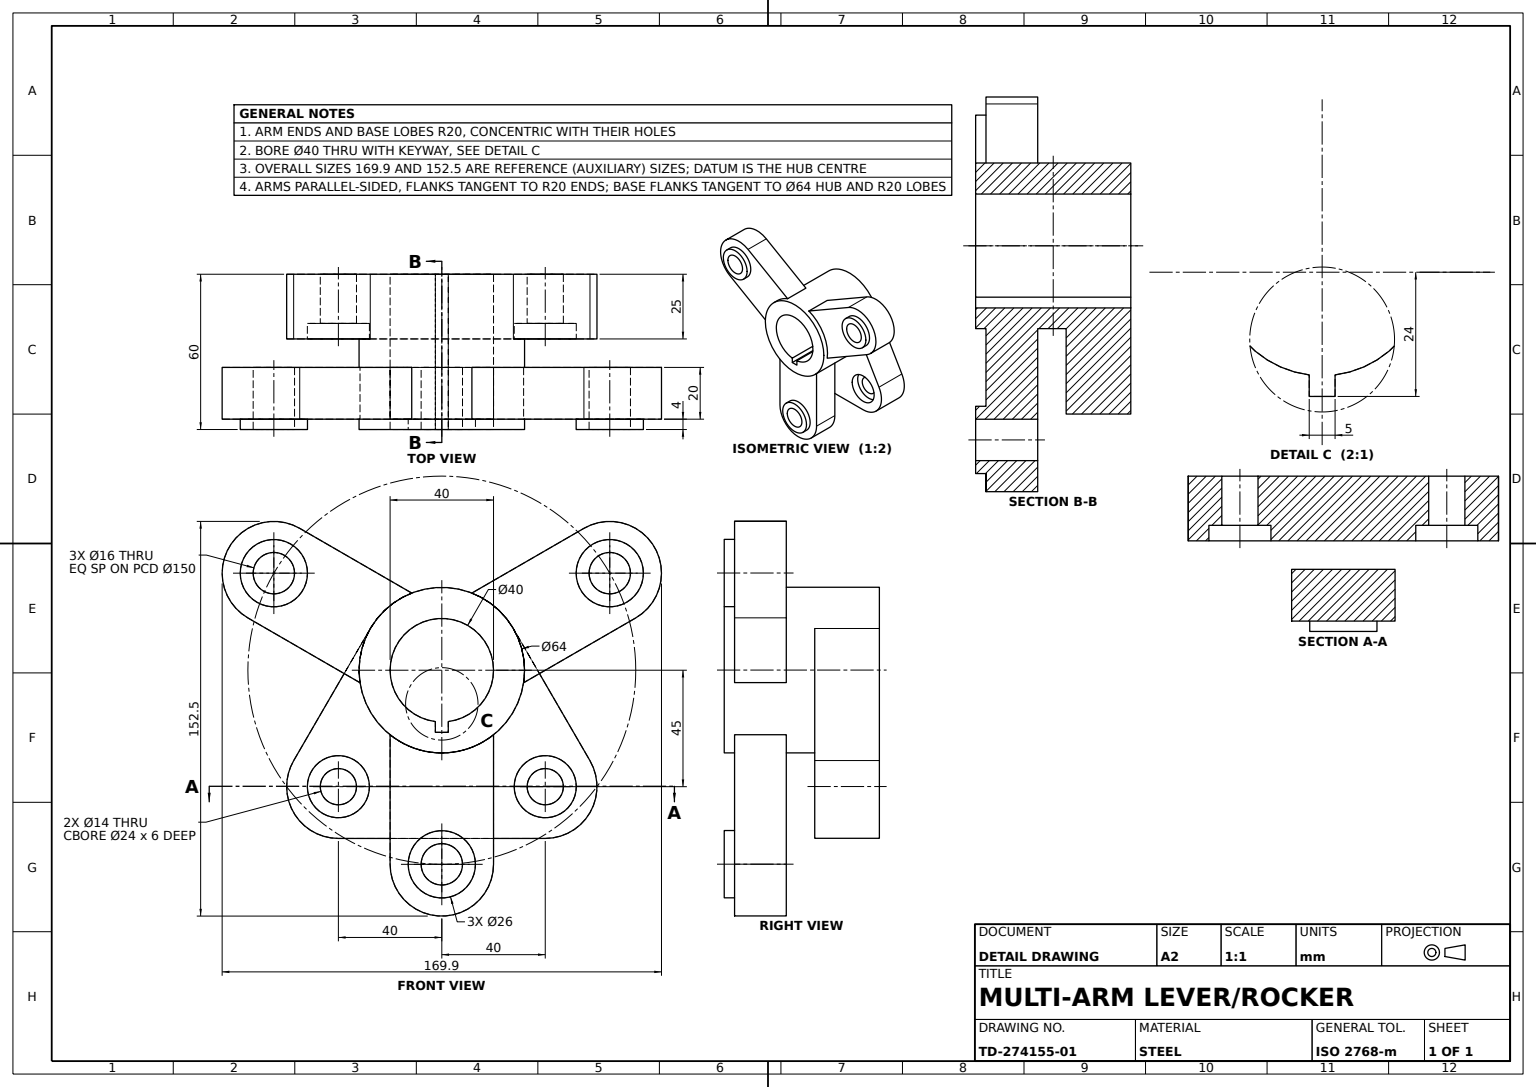
from build123d import *

# Parameters (mm, degrees)
BASE_BLOCK_DEPTH            = 25
HUB_SKETCH_64_R             = 32
HUB_64_DEPTH                = 31
THREE_START                 = -20
THREE_ARMS_120DEG_DEPTH     = 20
HUB_COLLAR_SKETCH_64_R      = 32
HUB_COLLAR_64X4_DEPTH       = 4
BOLT_BOSSES_SKETCH_3X_13_R  = 13
BOLT_BOSSES_3X_13_DEPTH     = 4
BOLT_HOLES_SKETCH_3X_8_R    = 8
BOLT_HOLES_3X_8_DEPTH       = 25
KEYED_BORE_24_DEPTH         = 80
COUNTERBORE_SKETCH_2X_12_R  = 12
COUNTERBORES_2X_12X6_DEPTH  = 6
THROUGH_HOLES_SKETCH_2X_7_R = 7
THROUGH_HOLES_2X_7_DEPTH    = 50


with BuildPart() as part:
    # Base Block Sketch → Base Block (new body)
    with BuildSketch(Plane.XY):
        with BuildLine():
            Line((-57.296551724, -34.95862069), (-27.674482759, 16.066206897))
            ThreePointArc((-27.674482759, 16.066206897), (0, 32), (27.674482759, 16.066206897))
            Line((27.674482759, 16.066206897), (57.296551724, -34.95862069))
            ThreePointArc((57.296551724, -34.95862069), (57.332449137, -54.979288897), (40, -65))
            Line((40, -65), (-40, -65))
            ThreePointArc((-40, -65), (-57.332449137, -54.979288897), (-57.296551724, -34.95862069))
        make_face()
    extrude(amount=BASE_BLOCK_DEPTH)

    # Hub Sketch _64 → Hub _64 (add)
    with BuildSketch(Plane.XY.offset(25)):
        with Locations(Location((0, 0, 0), (0, 0, 149.863023681))):
            Circle(HUB_SKETCH_64_R)
    extrude(amount=HUB_64_DEPTH)

    # Three Arms Sketch → Three Arms 120deg (add)
    with BuildSketch(Plane.XY.offset(56).offset(THREE_START)):
        with BuildLine():
            Line((-20, -75), (-20, -24.979991994))
            ThreePointArc((-20, -24.979991994), (0, -32), (20, -24.979991994))
            Line((20, -24.979991994), (20, -75))
            ThreePointArc((20, -75), (0, -95), (-20, -75))
        make_face()
        with BuildLine():
            Line((-11.633307653, 29.810504072), (-54.951905284, 54.820508076))
            ThreePointArc((-54.951905284, 54.820508076), (-82.27241336, 47.5), (-74.951905284, 20.179491924))
            Line((-74.951905284, 20.179491924), (-31.633307653, -4.830512079))
            ThreePointArc((-31.633307653, -4.830512079), (-27.712812921, 16), (-11.633307653, 29.810504072))
        make_face()
        with BuildLine():
            Line((17.280738855, 33.071049997), (54.951905284, 54.820508076))
            ThreePointArc((54.951905284, 54.820508076), (82.27146994, 47.501633873), (74.955172941, 20.181378918))
            Line((74.955172941, 20.181378918), (37.758368932, -1.303564067))
            Line((37.758368932, -1.303564067), (31.631479851, -4.842466563))
            ThreePointArc((31.631479851, -4.842466563), (27.715835779, 15.994763115), (11.633307653, 29.810504072))
            Line((11.633307653, 29.810504072), (17.280738855, 33.071049997))
        make_face()
    extrude(amount=THREE_ARMS_120DEG_DEPTH)

    # Hub Collar Sketch _64 → Hub Collar _64x4 (add)
    with BuildSketch(Plane.XY.offset(56)):
        with Locations(Location((0, 0, 0), (0, 0, 149.863023681))):
            Circle(HUB_COLLAR_SKETCH_64_R)
    extrude(amount=HUB_COLLAR_64X4_DEPTH)

    # Bolt Bosses Sketch 3x_13 → Bolt Bosses 3x_13 (add)
    with BuildSketch(Plane.XY.offset(56)):
        with Locations((-64.951905284, 37.5)):
            Circle(BOLT_BOSSES_SKETCH_3X_13_R)
        with Locations((64.951905284, 37.5)):
            Circle(BOLT_BOSSES_SKETCH_3X_13_R)
        with Locations((0, -75)):
            Circle(BOLT_BOSSES_SKETCH_3X_13_R)
    extrude(amount=BOLT_BOSSES_3X_13_DEPTH)

    # Bolt Holes Sketch 3x_8 → Bolt Holes 3x_8 (cut)
    with BuildSketch(Plane.XY.offset(60)):
        with Locations((-64.951905284, 37.5)):
            Circle(BOLT_HOLES_SKETCH_3X_8_R)
        with Locations((64.951905284, 37.5)):
            Circle(BOLT_HOLES_SKETCH_3X_8_R)
        with Locations((0, -75)):
            Circle(BOLT_HOLES_SKETCH_3X_8_R)
    extrude(amount=-BOLT_HOLES_3X_8_DEPTH, mode=Mode.SUBTRACT)

    # Keyed Bore Sketch _24 → Keyed Bore _24 (cut)
    with BuildSketch(Plane.XY.offset(60)):
        with BuildLine():
            Line((2.5, -24), (-2.5, -24))
            Line((-2.5, -24), (-2.5, -19.843134833))
            ThreePointArc((-2.5, -19.843134833), (0, 20), (2.5, -19.843134833))
            Line((2.5, -19.843134833), (2.5, -24))
        make_face()
    extrude(amount=-KEYED_BORE_24_DEPTH, mode=Mode.SUBTRACT)

    # Counterbore Sketch 2x_12 → Counterbores 2x_12x6 (cut)
    with BuildSketch(Plane.XY.offset(25)):
        with Locations((-40, -45)):
            Circle(COUNTERBORE_SKETCH_2X_12_R)
        with Locations((40, -45)):
            Circle(COUNTERBORE_SKETCH_2X_12_R)
    extrude(amount=-COUNTERBORES_2X_12X6_DEPTH, mode=Mode.SUBTRACT)

    # Through Holes Sketch 2x_7 → Through Holes 2x_7 (cut)
    with BuildSketch(Plane.XY.offset(19)):
        with Locations((-40, -45)):
            Circle(THROUGH_HOLES_SKETCH_2X_7_R)
        with Locations((40, -45)):
            Circle(THROUGH_HOLES_SKETCH_2X_7_R)
    extrude(amount=-THROUGH_HOLES_2X_7_DEPTH, mode=Mode.SUBTRACT)


solid = part.part
